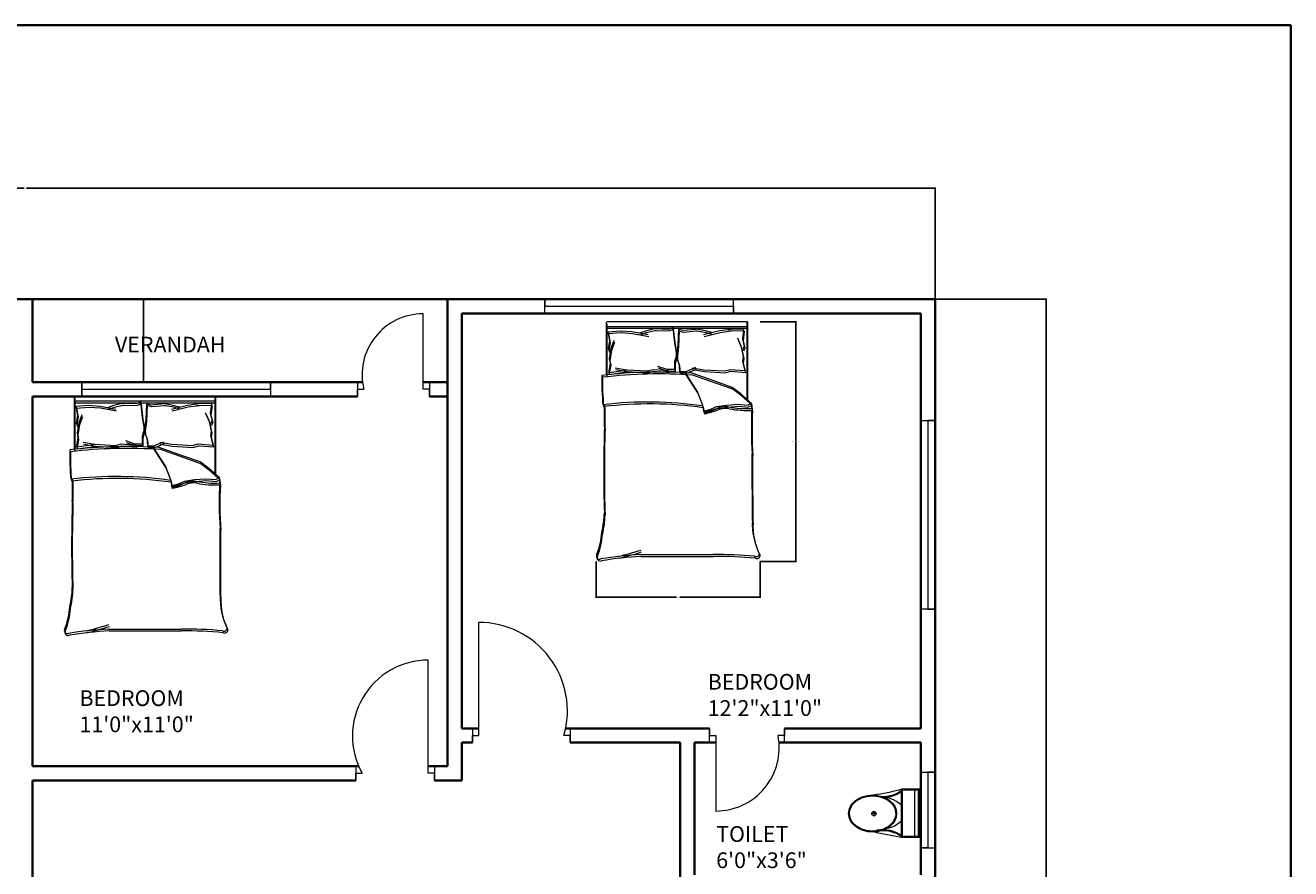
# Model space of a CAD drawing. Units: inches. Extents: x 2234 to 3001, y 1541 to 2386.
# Tile 12 of 12: x 2599 to 3001, y 2118 to 2386. Entities that reach past the tile are written whole.
import ezdxf

# ---------------------------------------------------------------- set-up
doc = ezdxf.new("R2010")
doc.units = ezdxf.units.IN
for name, color, linetype, lineweight in [('A-ANNO-DIMS', 2, 'Continuous', 18), ('A-ANNO-TTLB', 7, 'Continuous', 35), ('A-AREA-IDEN', 7, 'Continuous', 18), ('A-DOOR', 3, 'Continuous', 18), ('A-FLOR-FIXT', 9, 'Continuous', 18), ('A-FURN', 9, 'Continuous', 13), ('A-GLAZ', 4, 'Continuous', 18), ('A-WALL', 7, 'Continuous', 35)]:
    doc.layers.add(name, color=color, linetype=linetype, lineweight=lineweight)
doc.styles.get("Standard").update_dxf_attribs({"font": 'arial.ttf'})
doc.dimstyles.get("Standard").update_dxf_attribs({"dimtxt": 0.18, "dimasz": 0.18, "dimexe": 0.18, "dimexo": 0.0625, "dimgap": 0.09, "dimtad": 0, "dimtih": 1, "dimtoh": 1, "dimdec": 4, "dimzin": 0, "dimdsep": 46, "dimtxsty": 'Standard', "dimcen": 0.09, "dimadec": 0, "dimazin": 0, "dimtfac": 1, "dimtdec": 4, "dimtofl": 0, "dimtmove": 0, "dimatfit": 3, "dimfxl": 1, "dimtolj": 1, "dimtzin": 0, "dimarcsym": 0})

# ---------------------------------------------------------------- blocks, each defined once
blk = doc.blocks.new('A$C31115884')
for p, q in [((283, 498), (223, 498)), ((258, 466), (258, 523)), ((0, 200), (0, 0)), ((520, 200), (0, 200)), ((10, 190), (10, 10)), ((510, 190), (10, 190)), ((510, 10), (510, 190)), ((520, 0), (520, 200)), ((510, 54), (0, 54)), ((10, 10), (510, 10)), ((0, 0), (520, 0))]:
    blk.add_line(p, q)
blk.add_circle((256, 496), 23.6)
for centre, radius, start, end in [((2778, -205), 2807, 165.4549, 171.7133), ((-295, 403), 365, 324.2091, 9.3499), ((-295, 403), 375, 324.2091, 9.3499), ((139, 406), 293, 315.8436, 2.6563), ((806, 403), 365, 170.6501, 215.7909), ((3237, 905), 2807, 188.2867, 194.5451), ((384, 406), 293, 190.2774, 224.1564), ((806, 403), 375, 179.2036, 215.7909)]:
    blk.add_arc(centre, radius, start, end)
blk.add_ellipse((256, 510), major_axis=(0, -261), ratio=0.772727)
blk.add_open_spline([(256, 259), (263, 259), (270, 260), (288, 262), (299, 265), (320, 273), (330, 278), (350, 291), (360, 299), (378, 316), (386, 326), (402, 347), (409, 358), (421, 383), (427, 395), (436, 422), (440, 436), (445, 465), (447, 480), (448, 509), (448, 524), (445, 553), (443, 568), (436, 596), (432, 610), (422, 636), (416, 649), (402, 672), (395, 683), (379, 703), (370, 712), (351, 728), (341, 735), (321, 746), (310, 751), (289, 757), (278, 759), (256, 761), (245, 761), (223, 757), (212, 754), (191, 746), (181, 741), (161, 728), (151, 720), (133, 703), (125, 693), (110, 672), (103, 660), (90, 636), (85, 623), (76, 596), (72, 582), (67, 553), (66, 538), (64, 509), (65, 494), (68, 465), (70, 450), (77, 422), (81, 408), (91, 382), (97, 370), (111, 346), (118, 335), (135, 316), (144, 307), (162, 291), (172, 284), (193, 273), (203, 269), (225, 262), (236, 260), (250, 259), (253, 259), (256, 259)], degree=3, knots=[0, 0, 0, 0, 0.110105, 0.110105, 0.285049, 0.285049, 0.459994, 0.459994, 0.634938, 0.634938, 0.809882, 0.809882, 0.984827, 0.984827, 1.159771, 1.159771, 1.334715, 1.334715, 1.50966, 1.50966, 1.684604, 1.684604, 1.859549, 1.859549, 2.034493, 2.034493, 2.209437, 2.209437, 2.384382, 2.384382, 2.559326, 2.559326, 2.73427, 2.73427, 2.909215, 2.909215, 3.084159, 3.084159, 3.259103, 3.259103, 3.434048, 3.434048, 3.608992, 3.608992, 3.783936, 3.783936, 3.958881, 3.958881, 4.133825, 4.133825, 4.30877, 4.30877, 4.483714, 4.483714, 4.658658, 4.658658, 4.833603, 4.833603, 5.008547, 5.008547, 5.183491, 5.183491, 5.358436, 5.358436, 5.53338, 5.53338, 5.708324, 5.708324, 5.883269, 5.883269, 6.058213, 6.058213, 6.233158, 6.233158, 6.283185, 6.283185, 6.283185, 6.283185])
blk = doc.blocks.new('WIN-60-A')
for p, q in [((0, 60), (4.5, 60)), ((4.5, 60), (2.25, 60)), ((2.25, 60), (2.25, 0)), ((2.25, 0), (0, 0)), ((0, 0), (4.5, 0))]:
    blk.add_line(p, q)
blk = doc.blocks.new('WIN-24-A')
for p, q in [((0, 24), (4.5, 24)), ((4.5, 24), (2.25, 24)), ((2.25, 24), (2.25, 0)), ((2.25, 0), (0, 0)), ((0, 0), (4.5, 0))]:
    blk.add_line(p, q)
blk = doc.blocks.new('WIN-60-B')
for p, q in [((0, 60), (4.5, 60)), ((4.5, 60), (2.25, 60)), ((2.25, 60), (2.25, 0)), ((4.5, 0), (0, 0)), ((2.25, 0), (4.5, 0))]:
    blk.add_line(p, q)
blk = doc.blocks.new('BED-DOUBLE-A')
for p, q in [((3.24, 59.14), (3.24, 76.05)), ((3.24, 59.14), (3.24, 76.05)), ((3.24, 74.62), (47.87, 74.62)), ((3.24, 74.62), (47.87, 74.62)), ((48.08, 76.05), (3.46, 76.05)), ((3.46, 58.54), (3.46, 75.45)), ((3.46, 58.54), (3.46, 75.45)), ((3.46, 74.02), (48.08, 74.02)), ((3.46, 74.02), (48.08, 74.02)), ((3.64, 72.93), (7.64, 73.24)), ((3.64, 72.93), (7.64, 73.24)), ((3.64, 72.95), (4.18, 69.98)), ((3.64, 72.95), (4.18, 69.98)), ((3.85, 72.33), (7.85, 72.64)), ((3.85, 72.33), (7.85, 72.64)), ((7.64, 73.24), (7.74, 73.22)), ((7.64, 73.24), (7.74, 73.22)), ((7.74, 73.22), (11.31, 72.95)), ((7.74, 73.22), (11.31, 72.95)), ((7.85, 72.64), (7.95, 72.62)), ((7.85, 72.64), (7.95, 72.62)), ((7.95, 72.62), (11.52, 72.35)), ((7.95, 72.62), (11.52, 72.35)), ((11.31, 72.95), (16.44, 72.01)), ((11.31, 72.95), (16.44, 72.01)), ((13.87, 72.55), (15.76, 73.22)), ((13.87, 72.55), (15.76, 73.22)), ((14.08, 71.95), (15.97, 72.62)), ((14.08, 71.95), (15.97, 72.62)), ((15.76, 73.22), (18.46, 73.9)), ((15.76, 73.22), (18.46, 73.9)), ((15.97, 72.62), (18.67, 73.3)), ((15.97, 72.62), (18.67, 73.3)), ((18.46, 73.9), (18.76, 73.9)), ((18.46, 73.9), (18.76, 73.9)), ((18.67, 73.3), (18.97, 73.3)), ((18.67, 73.3), (18.97, 73.3)), ((18.76, 73.9), (22.91, 73.76)), ((18.76, 73.9), (22.91, 73.76)), ((18.97, 73.3), (23.12, 73.16)), ((18.97, 73.3), (23.12, 73.16)), ((22.91, 73.76), (24.26, 74.3)), ((22.91, 73.76), (24.26, 74.3)), ((23.12, 73.16), (24.47, 73.7)), ((23.12, 73.16), (24.47, 73.7)), ((24.26, 74.3), (24.8, 69.31)), ((24.26, 74.3), (24.8, 69.31)), ((24.47, 73.7), (25.01, 68.71)), ((24.47, 73.7), (25.01, 68.71)), ((26.12, 73.72), (25.9, 68.7)), ((26.12, 73.72), (25.9, 68.7)), ((26.34, 73.12), (26.11, 68.1)), ((26.34, 73.12), (26.11, 68.1)), ((27.5, 73.27), (26.12, 73.72)), ((27.5, 73.27), (26.12, 73.72)), ((27.72, 72.67), (26.34, 73.12)), ((27.72, 72.67), (26.34, 73.12)), ((31.64, 73.66), (27.5, 73.27)), ((31.64, 73.66), (27.5, 73.27)), ((31.85, 73.06), (27.72, 72.67)), ((31.85, 73.06), (27.72, 72.67)), ((31.94, 73.68), (31.64, 73.66)), ((31.94, 73.68), (31.64, 73.66)), ((32.15, 73.08), (31.85, 73.06)), ((32.15, 73.08), (31.85, 73.06)), ((34.67, 73.17), (31.94, 73.68)), ((34.67, 73.17), (31.94, 73.68)), ((34.89, 72.58), (32.15, 73.08)), ((34.89, 72.58), (32.15, 73.08)), ((39.14, 73.18), (34.08, 71.92)), ((39.14, 73.18), (34.08, 71.92)), ((39.35, 72.58), (34.29, 71.32)), ((39.35, 72.58), (34.29, 71.32)), ((36.6, 72.62), (34.67, 73.17)), ((36.6, 72.62), (34.67, 73.17)), ((36.82, 72.02), (34.89, 72.58)), ((36.82, 72.02), (34.89, 72.58)), ((42.68, 73.67), (39.14, 73.18)), ((42.68, 73.67), (39.14, 73.18)), ((42.9, 73.08), (39.35, 72.58)), ((42.9, 73.08), (39.35, 72.58)), ((46.79, 73.66), (41.75, 73.75)), ((41.75, 73.75), (42.68, 73.67)), ((46.79, 73.66), (41.75, 73.75)), ((41.75, 73.75), (42.68, 73.67)), ((47.01, 73.06), (41.96, 73.15)), ((41.96, 73.15), (42.9, 73.08)), ((47, 73.06), (41.96, 73.15)), ((41.96, 73.15), (42.9, 73.08)), ((46.79, 73.66), (46.44, 70.66)), ((46.79, 73.66), (46.44, 70.66)), ((47.01, 73.06), (46.65, 70.07)), ((47, 73.06), (46.65, 70.07)), ((47.87, 76.05), (47.87, 51.2)), ((47.87, 76.05), (47.87, 51.2)), ((48.08, 76.05), (48.08, 75.45)), ((48.08, 75.45), (48.08, 50.6)), ((48.08, 75.45), (48.08, 50.6)), ((4.18, 69.98), (3.77, 67.55)), ((4.18, 69.98), (3.77, 67.55)), ((3.85, 72.35), (4.39, 69.38)), ((3.85, 72.35), (4.39, 69.38)), ((4.39, 69.38), (3.98, 66.95)), ((4.39, 69.38), (3.98, 66.95)), ((4.72, 67.69), (5.66, 70.25)), ((4.72, 67.69), (5.66, 70.25)), ((4.93, 67.09), (5.87, 69.65)), ((4.93, 67.09), (5.87, 69.65)), ((11.52, 72.35), (16.65, 71.41)), ((11.52, 72.35), (16.65, 71.41)), ((24.8, 69.31), (25.34, 66.34)), ((24.8, 69.31), (25.34, 66.34)), ((25.01, 68.71), (25.55, 65.74)), ((25.01, 68.71), (25.55, 65.74)), ((25.9, 68.7), (25.54, 65.7)), ((25.9, 68.7), (25.54, 65.7)), ((46.04, 68.34), (44.94, 70.84)), ((46.04, 68.34), (44.94, 70.84)), ((46.26, 67.74), (45.15, 70.24)), ((46.26, 67.74), (45.15, 70.24)), ((46.44, 70.66), (46.99, 68.26)), ((46.44, 70.66), (46.99, 68.26)), ((46.65, 70.07), (47.21, 67.66)), ((46.65, 70.07), (47.21, 67.66)), ((3.77, 67.55), (4.31, 66.61)), ((3.77, 67.55), (4.31, 66.61)), ((3.98, 66.95), (4.52, 66.01)), ((3.98, 66.95), (4.52, 66.01)), ((4.18, 64.31), (4.72, 67.69)), ((4.18, 64.31), (4.72, 67.69)), ((4.39, 63.71), (4.93, 67.09)), ((4.39, 63.71), (4.93, 67.09)), ((25.34, 65.12), (24.8, 63.37)), ((25.34, 65.12), (24.8, 63.37)), ((25.55, 64.52), (25.01, 62.77)), ((25.55, 64.52), (25.01, 62.77)), ((25.34, 66.34), (25.34, 65.12)), ((25.34, 66.34), (25.34, 65.12)), ((25.54, 65.7), (25.62, 64.49)), ((25.54, 65.7), (25.62, 64.49)), ((25.55, 65.74), (25.55, 64.52)), ((25.55, 65.74), (25.55, 64.52)), ((25.62, 64.49), (26.27, 62.77)), ((25.62, 64.49), (26.27, 62.77)), ((26.11, 68.1), (25.76, 65.11)), ((26.11, 68.1), (25.76, 65.11)), ((25.76, 65.11), (25.83, 63.89)), ((25.76, 65.11), (25.83, 63.89)), ((46.79, 65), (46.04, 68.34)), ((46.79, 65), (46.04, 68.34)), ((47.01, 64.41), (46.26, 67.74)), ((47, 64.41), (46.26, 67.74)), ((46.99, 68.26), (46.51, 67.28)), ((46.99, 68.26), (46.51, 67.28)), ((46.61, 63.5), (46.79, 65)), ((46.62, 63.5), (46.79, 65)), ((47.21, 67.66), (46.73, 66.69)), ((47.21, 67.66), (46.73, 66.69)), ((46.83, 62.91), (47.01, 64.41)), ((46.83, 62.91), (47, 64.41)), ((3.91, 59.86), (4.45, 62.83)), ((3.91, 59.86), (4.45, 62.83)), ((8.67, 60.53), (3.91, 59.86)), ((8.67, 60.53), (3.91, 59.86)), ((4.12, 59.26), (4.66, 62.23)), ((4.12, 59.26), (4.66, 62.23)), ((4.45, 62.83), (4.18, 64.31)), ((4.45, 62.83), (4.18, 64.31)), ((4.66, 62.23), (4.39, 63.71)), ((4.66, 62.23), (4.39, 63.71)), ((5.96, 61.45), (9.72, 60.83)), ((5.96, 61.45), (9.72, 60.83)), ((6.17, 60.86), (9.94, 60.24)), ((6.17, 60.86), (9.94, 60.24)), ((9.72, 60.83), (8.67, 60.53)), ((9.72, 60.83), (8.67, 60.53)), ((9.72, 60.83), (16.27, 60.43)), ((9.72, 60.83), (16.27, 60.43)), ((16.27, 60.43), (18.1, 60.95)), ((16.27, 60.43), (18.1, 60.95)), ((16.48, 59.83), (18.31, 60.35)), ((16.48, 59.83), (18.31, 60.35)), ((18.1, 60.95), (22.89, 60.57)), ((18.1, 60.95), (22.89, 60.57)), ((18.31, 60.35), (23.1, 59.98)), ((18.31, 60.35), (23.1, 59.98)), ((22.51, 60.86), (19.57, 61.88)), ((22.51, 60.86), (19.57, 61.88)), ((22.72, 60.27), (19.78, 61.28)), ((22.72, 60.27), (19.78, 61.28)), ((24.8, 60.86), (22.51, 60.86)), ((24.8, 60.86), (22.51, 60.86)), ((24.8, 63.37), (24.8, 60.86)), ((24.8, 63.37), (24.8, 60.86)), ((25.01, 62.77), (25.01, 60.27)), ((25.01, 62.77), (25.01, 60.27)), ((25.83, 63.89), (26.48, 62.18)), ((25.83, 63.89), (26.48, 62.18)), ((26.27, 62.77), (26.42, 60.27)), ((26.27, 62.77), (26.42, 60.27)), ((26.42, 60.27), (28.71, 60.42)), ((26.42, 60.27), (28.71, 60.42)), ((26.48, 62.18), (26.64, 59.68)), ((26.48, 62.18), (26.64, 59.68)), ((28.71, 60.42), (31.58, 61.62)), ((28.71, 60.42), (31.58, 61.62)), ((28.93, 59.82), (31.79, 61.02)), ((28.93, 59.82), (31.79, 61.02)), ((30.41, 61.45), (34.17, 60.83)), ((30.41, 61.45), (34.17, 60.83)), ((30.62, 60.86), (34.38, 60.24)), ((30.62, 60.86), (34.38, 60.24)), ((34.17, 60.83), (40.72, 60.43)), ((34.17, 60.83), (40.72, 60.43)), ((40.72, 60.43), (42.55, 60.95)), ((40.72, 60.43), (42.55, 60.95)), ((40.93, 59.83), (42.76, 60.35)), ((40.93, 59.83), (42.76, 60.35)), ((42.55, 60.95), (47.34, 60.57)), ((42.55, 60.95), (47.34, 60.57)), ((42.76, 60.35), (47.55, 59.98)), ((42.76, 60.35), (47.55, 59.98)), ((47.34, 60.57), (46.61, 63.5)), ((47.34, 60.57), (46.62, 63.5)), ((47.55, 59.98), (46.83, 62.91)), ((47.55, 59.98), (46.83, 62.91)), ((8.88, 59.93), (4.12, 59.26)), ((8.88, 59.93), (4.12, 59.26)), ((9.94, 60.24), (8.88, 59.93)), ((9.94, 60.24), (8.88, 59.93)), ((9.94, 60.24), (16.48, 59.83)), ((9.94, 60.24), (16.48, 59.83)), ((25.01, 60.27), (22.72, 60.27)), ((25.01, 60.27), (22.72, 60.27)), ((26.64, 59.68), (28.93, 59.82)), ((26.64, 59.68), (28.93, 59.82)), ((28.25, 59.82), (32.17, 53.75)), ((28.25, 59.82), (32.17, 53.75)), ((28.47, 59.22), (32.38, 53.16)), ((28.47, 59.22), (32.38, 53.16)), ((37.95, 57.08), (30.17, 59.82)), ((37.95, 57.08), (30.17, 59.82)), ((38.16, 56.48), (30.38, 59.22)), ((38.16, 56.48), (30.38, 59.22)), ((34.38, 60.24), (40.93, 59.83)), ((34.38, 60.24), (40.93, 59.83)), ((43.16, 55.2), (37.95, 57.08)), ((43.16, 55.2), (37.95, 57.08)), ((43.37, 54.6), (38.16, 56.48)), ((43.37, 54.6), (38.16, 56.48)), ((32.17, 53.75), (33.76, 49.56)), ((32.17, 53.75), (33.76, 49.56)), ((32.38, 53.16), (33.97, 48.97)), ((32.38, 53.16), (33.97, 48.97)), ((45.91, 53.18), (43.16, 55.2)), ((45.9, 53.18), (43.16, 55.2)), ((46.12, 52.58), (43.37, 54.6)), ((46.12, 52.58), (43.37, 54.6)), ((49.36, 50.14), (45.9, 53.18)), ((49.37, 50.14), (45.91, 53.18)), ((49.58, 49.54), (46.12, 52.58)), ((49.58, 49.54), (46.12, 52.58)), ((33.76, 49.56), (34.05, 47.68)), ((33.76, 49.56), (34.05, 47.68)), ((33.97, 48.97), (34.26, 47.09)), ((33.97, 48.97), (34.26, 47.09)), ((36.36, 48.26), (38.24, 49.13)), ((36.36, 48.26), (38.24, 49.13)), ((36.57, 47.66), (38.45, 48.53)), ((36.57, 47.66), (38.45, 48.53)), ((38.24, 49.13), (41.42, 49.56)), ((38.24, 49.13), (41.42, 49.56)), ((38.45, 48.53), (41.64, 48.97)), ((38.45, 48.53), (41.64, 48.97)), ((41.42, 49.56), (45.04, 49.85)), ((41.42, 49.56), (45.04, 49.85)), ((41.64, 48.97), (45.25, 49.25)), ((41.64, 48.97), (45.25, 49.25)), ((45.04, 49.85), (47.93, 49.56)), ((45.04, 49.85), (47.93, 49.56)), ((45.25, 49.25), (48.14, 48.97)), ((45.25, 49.25), (48.14, 48.97)), ((47.93, 49.56), (49.37, 50.14)), ((47.93, 49.56), (49.36, 50.14)), ((48.14, 48.97), (49.58, 49.54)), ((48.14, 48.97), (49.58, 49.54)), ((49.44, 48.51), (49.36, 50.14, 3.61)), ((49.44, 48.51), (49.37, 50.14, 3.61)), ((49.65, 47.91), (49.58, 49.54, 3.61)), ((49.65, 47.91), (49.58, 49.54, 3.61)), ((34.05, 47.68), (36.36, 48.26)), ((34.05, 47.68), (36.36, 48.26)), ((34.26, 47.09), (36.57, 47.66)), ((34.26, 47.09), (36.57, 47.66)), ((14.07, 2.05), (37.05, 2.05)), ((14.07, 2.05), (37.05, 2.05)), ((14.28, 1.46), (37.26, 1.46)), ((14.28, 1.46), (37.26, 1.46))]:
    blk.add_line(p, q)
for centre, radius, start, end in [((79.52, 57.28), 77.79, 178.7218, 185.604), ((79.52, 57.28), 77.79, 178.7218, 185.604), ((19.94, -93.94), 154.04, 86.0865, 96.7821), ((19.94, -93.94), 154.04, 86.0865, 96.7821), ((79.73, 56.69), 77.79, 178.7218, 185.604), ((79.73, 56.69), 77.79, 178.7218, 185.604), ((20.16, -94.54), 154.04, 86.0865, 96.7821), ((20.16, -94.54), 154.04, 86.0865, 96.7821), ((16.58, -69.91), 120.47, 81.7845, 96.9006), ((16.58, -69.91), 120.47, 81.7845, 96.9006), ((16.79, -70.51), 120.47, 81.7845, 96.9006), ((16.79, -70.51), 120.47, 81.7845, 96.9006), ((-156.22, 46.94), 158.84, 358.4762, 1.0082), ((-156.22, 46.94), 158.84, 358.4762, 1.0082), ((-156.01, 46.34), 158.84, 358.4762, 1.0082), ((-156.01, 46.34), 158.84, 358.4762, 1.0082), ((29.09, 74.66), 27.69, 280.6617, 289.8806), ((29.09, 74.66), 27.69, 280.6617, 289.8806), ((40.85, 43.3), 5.81, 78.6608, 113.7384), ((40.85, 43.3), 5.81, 78.6608, 113.7384), ((41.06, 42.71), 5.81, 78.6608, 113.7384), ((41.06, 42.71), 5.81, 78.6608, 113.7384), ((47.93, 82.26), 33.79, 259.8763, 272.5657), ((47.93, 82.26), 33.79, 259.8763, 272.5657), ((48.14, 81.67), 33.79, 259.8763, 272.5657), ((48.14, 81.67), 33.79, 259.8763, 272.5657), ((170.19, 42.14), 120.92, 176.9791, 183.8365), ((170.19, 42.14), 120.92, 176.9791, 183.8365), ((34.21, 47.63), 0.172, 160.2464, 271.1377), ((34.21, 47.63), 0.172, 160.2464, 271.1377), ((34.42, 47.03), 0.172, 160.2464, 271.1377), ((34.42, 47.03), 0.172, 160.2464, 271.1377), ((29.3, 74.07), 27.69, 280.6617, 289.8806), ((29.3, 74.07), 27.69, 280.6617, 289.8806), ((170.4, 41.54), 120.92, 176.9791, 183.8365), ((170.4, 41.54), 120.92, 176.9791, 183.8365), ((452.7, 28.79), 450.36, 178.2277, 181.7185), ((452.7, 28.79), 450.36, 178.2277, 181.7185), ((452.91, 28.19), 450.36, 178.2277, 181.7185), ((452.91, 28.19), 450.36, 178.2277, 181.7185), ((-4210.02, 12.72), 4259.62, 0.00217, 0.28689), ((-4210.02, 12.72), 4259.62, 0.00217, 0.28689), ((-4209.81, 12.12), 4259.62, 0.00217, 0.28689), ((-4209.81, 12.12), 4259.62, 0.00217, 0.28689), ((-25.12, 15.81), 27.67, 346.0648, 358.9113), ((-25.12, 15.81), 27.67, 346.0648, 358.9113), ((-24.9, 15.21), 27.67, 346.0648, 358.9113), ((-24.9, 15.21), 27.67, 346.0648, 358.9113), ((71.11, 11.93), 21.54, 177.4714, 206.4681), ((71.11, 11.93), 21.54, 177.4714, 206.4681), ((71.32, 11.33), 21.54, 177.4714, 206.4681), ((71.32, 11.33), 21.54, 177.4714, 206.4681), ((-20.22, 10.43), 22, 337.9751, 356.652), ((-20.22, 10.43), 22, 337.9751, 356.652), ((-20.01, 9.83), 22, 337.9751, 356.652), ((-20.01, 9.83), 22, 337.9751, 356.652), ((1.02, 1.61), 1.02, 146.1736, 293.4781), ((1.02, 1.61), 1.02, 146.1736, 293.4781), ((1.23, 1.01), 1.02, 146.1736, 293.4781), ((1.23, 1.01), 1.02, 146.1736, 293.4781), ((20.01, -111.48), 113.69, 92.9958, 99.4091), ((20.01, -111.48), 113.69, 92.9958, 99.4091), ((20.22, -112.08), 113.69, 92.9958, 99.4091), ((20.22, -112.08), 113.69, 92.9958, 99.4091), ((-16.08, 98.19), 99.41, 283.3832, 287.7053), ((-16.08, 98.19), 99.41, 283.3832, 287.7053), ((-15.87, 97.59), 99.41, 283.3832, 287.7053), ((-15.87, 97.59), 99.41, 283.3832, 287.7053), ((38.43, -122.16), 124.23, 84.4998, 90.6351), ((38.43, -122.16), 124.23, 84.4998, 90.6351), ((38.64, -122.76), 124.23, 84.4998, 90.6351), ((38.64, -122.76), 124.23, 84.4998, 90.6351), ((50.81, 2.4), 1.03, 242.6588, 356.02), ((50.8, 2.4), 1.03, 242.6588, 356.02), ((51.02, 1.81), 1.03, 242.6588, 356.02), ((51.02, 1.81), 1.03, 242.6588, 356.02)]:
    blk.add_arc(centre, radius, start, end)
blk = doc.blocks.new('*D35')
at = {"layer": 'A-ANNO-DIMS', "color": 0, "lineweight": -2, "transparency": 16777216}
for p, q in [((2832.68, 2291.4), (2844.22, 2291.4)), ((2844.04, 2291.22), (2844.04, 2253.51)), ((2844.04, 2215.44), (2844.04, 2253.15)), ((2832.68, 2215.26), (2844.22, 2215.26))]:
    blk.add_line(p, q, dxfattribs=at)
at = {"layer": 'A-ANNO-DIMS', "color": 0, "transparency": 16777216}
for points in [[(2844.01, 2291.22), (2844.07, 2291.22), (2844.04, 2291.4)], [(2844.01, 2215.44), (2844.07, 2215.44), (2844.04, 2215.26)]]:
    blk.add_solid(points, dxfattribs=at)
at = {"layer": 'Defpoints', "color": 0, "transparency": 16777216}
for p in [(2832.62, 2291.4), (2844.04, 2291.4), (2832.62, 2215.26)]:
    blk.add_point(p, dxfattribs=at)
at = {"layer": 'A-ANNO-DIMS', "color": 0, "transparency": 16777216, "insert": (2844.04, 2253.33), "char_height": 0.18, "attachment_point": 5}
blk.add_mtext('\\A1;DOUBLE BED A 76 TYP.', dxfattribs=at)
blk = doc.blocks.new('*D36')
at = {"layer": 'A-ANNO-DIMS', "color": 0, "lineweight": -2, "transparency": 16777216}
for p, q in [((2780.49, 2215.19), (2780.49, 2203.66)), ((2832.62, 2215.19), (2832.62, 2203.66)), ((2780.67, 2203.84), (2806.03, 2203.84)), ((2832.44, 2203.84), (2807.09, 2203.84))]:
    blk.add_line(p, q, dxfattribs=at)
at = {"layer": 'A-ANNO-DIMS', "color": 0, "transparency": 16777216}
for points in [[(2780.67, 2203.87), (2780.67, 2203.81), (2780.49, 2203.84)], [(2832.44, 2203.87), (2832.44, 2203.81), (2832.62, 2203.84)]]:
    blk.add_solid(points, dxfattribs=at)
at = {"layer": 'Defpoints', "color": 0, "transparency": 16777216}
for p in [(2780.49, 2215.26), (2832.62, 2215.26), (2832.62, 2203.84)]:
    blk.add_point(p, dxfattribs=at)
at = {"layer": 'A-ANNO-DIMS', "color": 0, "transparency": 16777216, "insert": (2806.56, 2203.84), "char_height": 0.18, "attachment_point": 5}
blk.add_mtext('\\A1;52 TYP.', dxfattribs=at)
blk = doc.blocks.new('*D61')
at = {"layer": 'A-ANNO-DIMS', "color": 0, "lineweight": -2, "transparency": 16777216}
for p, q in [((2309.75, 2298.67), (2309.75, 2334.14)), ((2309.93, 2333.96), (2598.61, 2333.96)), ((2888.07, 2333.96), (2599.4, 2333.96)), ((2888.25, 2298.67), (2888.25, 2334.14))]:
    blk.add_line(p, q, dxfattribs=at)
at = {"layer": 'A-ANNO-DIMS', "color": 0, "transparency": 16777216}
for points in [[(2309.93, 2333.99), (2309.93, 2333.93), (2309.75, 2333.96)], [(2888.07, 2333.99), (2888.07, 2333.93), (2888.25, 2333.96)]]:
    blk.add_solid(points, dxfattribs=at)
at = {"layer": 'Defpoints', "color": 0, "transparency": 16777216}
for p in [(2888.25, 2333.96), (2309.75, 2298.61), (2888.25, 2298.61)]:
    blk.add_point(p, dxfattribs=at)
at = {"layer": 'A-ANNO-DIMS', "color": 0, "transparency": 16777216, "insert": (2599, 2333.96), "char_height": 0.18, "attachment_point": 5}
blk.add_mtext('\\A1;578.5', dxfattribs=at)
blk = doc.blocks.new('*D62')
at = {"layer": 'A-ANNO-DIMS', "color": 0, "lineweight": -2, "transparency": 16777216}
for p, q in [((2888.32, 2298.61), (2923.78, 2298.61)), ((2923.6, 2298.43), (2923.6, 2000.54)), ((2923.6, 1702.29), (2923.6, 2000.18)), ((2888.32, 1702.11), (2923.78, 1702.11))]:
    blk.add_line(p, q, dxfattribs=at)
at = {"layer": 'A-ANNO-DIMS', "color": 0, "transparency": 16777216}
for points in [[(2923.57, 2298.43), (2923.63, 2298.43), (2923.6, 2298.61)], [(2923.57, 1702.29), (2923.63, 1702.29), (2923.6, 1702.11)]]:
    blk.add_solid(points, dxfattribs=at)
at = {"layer": 'Defpoints', "color": 0, "transparency": 16777216}
for p in [(2888.25, 2298.61), (2923.6, 2298.61), (2888.25, 1702.11)]:
    blk.add_point(p, dxfattribs=at)
at = {"layer": 'A-ANNO-DIMS', "color": 0, "transparency": 16777216, "insert": (2923.6, 2000.36), "char_height": 0.18, "attachment_point": 5}
blk.add_mtext('\\A1;596.5', dxfattribs=at)
blk = doc.blocks.new('*D67')
at = {"layer": 'A-ANNO-DIMS', "color": 0, "lineweight": -2, "transparency": 16777216}
for p, q in [((2601.32, 2298.61), (2636.78, 2298.61)), ((2636.6, 2298.43), (2636.6, 2285.6)), ((2636.6, 2272.4), (2636.6, 2285.23)), ((2601.32, 2272.22), (2636.78, 2272.22))]:
    blk.add_line(p, q, dxfattribs=at)
at = {"layer": 'A-ANNO-DIMS', "color": 0, "transparency": 16777216}
for points in [[(2636.57, 2298.43), (2636.63, 2298.43), (2636.6, 2298.61)], [(2636.57, 2272.4), (2636.63, 2272.4), (2636.6, 2272.22)]]:
    blk.add_solid(points, dxfattribs=at)
at = {"layer": 'Defpoints', "color": 0, "transparency": 16777216}
for p in [(2601.25, 2298.61), (2601.25, 2272.22), (2636.6, 2272.22)]:
    blk.add_point(p, dxfattribs=at)
at = {"layer": 'A-ANNO-DIMS', "color": 0, "transparency": 16777216, "insert": (2636.6, 2285.41), "char_height": 0.18, "attachment_point": 5}
blk.add_mtext('\\A1;26.39', dxfattribs=at)

msp = doc.modelspace()

# ---------------------------------------------------------------- linework, layer by layer
at = {"layer": 'A-ANNO-TTLB'}
msp.add_lwpolyline([(2233.5367, 2385.7012), (3001.3383, 2385.7012), (3001.3383, 1541.435), (2233.5367, 1541.435)], close=True, dxfattribs=at)
at = {"layer": 'A-DOOR'}
for p, q in [((2725.479, 2269.9685), (2725.479, 2293.9685)), ((2704.6613, 2272.2185), (2704.6613, 2267.7185)), ((2704.6613, 2267.7185), (2704.6613, 2269.9685)), ((2704.6613, 2269.9685), (2706.6613, 2269.9685)), ((2727.479, 2269.9685), (2725.479, 2269.9685)), ((2727.479, 2272.2185), (2727.479, 2267.7185)), ((2727.479, 2267.7185), (2727.479, 2269.9685)), ((2743.1877, 2159.861), (2743.1877, 2195.861)), ((2727.1204, 2147.861), (2727.1204, 2183.861)), ((2741.1877, 2162.111), (2741.1877, 2157.611)), ((2772.2799, 2162.111), (2772.2799, 2157.611)), ((2816.5683, 2157.611), (2816.5683, 2162.111)), ((2816.5683, 2162.111), (2816.5683, 2159.861)), ((2840.3413, 2157.611), (2840.3413, 2162.111)), ((2840.3413, 2162.111), (2840.3413, 2159.861)), ((2741.1877, 2157.611), (2741.1877, 2159.861)), ((2741.1877, 2159.861), (2743.1877, 2159.861)), ((2741.1877, 2157.611), (2741.1877, 2157.611)), ((2772.2799, 2159.861), (2770.2799, 2159.861)), ((2772.2799, 2157.611), (2772.2799, 2159.861)), ((2816.5683, 2159.861), (2818.5683, 2159.861)), ((2818.5683, 2159.861), (2818.5683, 2135.861)), ((2840.3413, 2159.861), (2838.3413, 2159.861)), ((2704.1426, 2150.111), (2704.1426, 2145.611)), ((2729.1204, 2150.111), (2729.1204, 2145.611)), ((2704.1426, 2145.611), (2704.1426, 2147.861)), ((2704.1426, 2147.861), (2706.1426, 2147.861)), ((2729.1204, 2147.861), (2727.1204, 2147.861)), ((2729.1204, 2145.611), (2729.1204, 2147.861))]:
    msp.add_line(p, q, dxfattribs=at)
for centre, radius, start, end in [((2725.479, 2274.5913), 19.3772, 90, 193.802081), ((2743.1877, 2167.6667), 28.1943, 343.927438, 90), ((2727.1204, 2159.7489), 24.1121, 90, 209.539718), ((2818.5683, 2156.0063), 20.1452, 270, 11.031501)]:
    msp.add_arc(centre, radius, start, end, dxfattribs=at)
at = {"layer": 'A-GLAZ'}
msp.add_line((2616.9992, 2272.2185), (2616.9992, 2267.7185), dxfattribs=at)
at = {"layer": 'A-WALL'}
for p, q in [((2464.7534, 2298.611), (2733.2534, 2298.611)), ((2596.7534, 2298.611), (2601.2534, 2298.611)), ((2601.2534, 2298.611), (2601.2534, 2272.2185)), ((2733.2534, 2298.611), (2733.2534, 2157.611)), ((2733.2534, 2298.611), (2888.2534, 2298.611)), ((2888.2534, 2298.611), (2888.2534, 1702.111)), ((2737.7534, 2294.111), (2737.7534, 2162.111)), ((2737.7534, 2294.111), (2883.7534, 2294.111)), ((2883.7534, 2294.111), (2883.7534, 2162.111)), ((2733.2534, 2282.111), (2733.2534, 2150.111)), ((2601.2534, 2277.611), (2601.2534, 2272.2185)), ((2601.2534, 2272.2185), (2706.2476, 2272.2185)), ((2725.479, 2272.2185), (2733.2534, 2272.2185)), ((2601.2534, 2267.7185), (2704.6613, 2267.7185)), ((2601.2534, 2267.7185), (2601.2534, 2150.111)), ((2727.479, 2267.7185), (2733.2534, 2267.7185)), ((2737.7534, 2162.111), (2743.1877, 2162.111)), ((2770.8292, 2162.111), (2816.5683, 2162.111)), ((2811.7534, 2162.111), (2807.2534, 2162.111)), ((2840.3413, 2162.111), (2883.7534, 2162.111)), ((2737.7534, 2157.611), (2741.1877, 2157.611)), ((2737.7534, 2145.611), (2737.7534, 2157.611)), ((2772.2799, 2157.611), (2807.2534, 2157.611)), ((2807.2534, 2157.611), (2807.2534, 2107.6086)), ((2811.7534, 2157.611), (2818.5683, 2157.611)), ((2811.7534, 2115.611), (2811.7534, 2157.611)), ((2838.6495, 2157.611), (2883.7534, 2157.611)), ((2883.7534, 2157.611), (2883.7534, 2115.611)), ((2705.0183, 2150.111), (2601.2534, 2150.111)), ((2733.2534, 2150.111), (2727.1204, 2150.111)), ((2601.2534, 2145.611), (2704.1426, 2145.611)), ((2601.2534, 2145.611), (2601.2534, 2004.611)), ((2729.1204, 2145.611), (2737.7534, 2145.611))]:
    msp.add_line(p, q, dxfattribs=at)

# ---------------------------------------------------------------- block references
at = {"layer": 'A-FLOR-FIXT', "xscale": 0.0292470664339069, "yscale": 0.0292470664339069, "zscale": 0.0292470664339069, "rotation": 89.99999999999999}
msp.add_blockref('A$C31115884', (2883.3221, 2127.5818), dxfattribs=at)
at = {"layer": 'A-FURN'}
for p in [(2780.5758, 2215.3549), (2611.3897, 2191.6708)]:
    msp.add_blockref('BED-DOUBLE-A', p, dxfattribs=at)
at = {"layer": 'A-GLAZ', "rotation": 90}
for name, p in [('WIN-60-A', (2824.1492, 2294.1106)), ('WIN-60-B', (2676.9995, 2267.7181))]:
    msp.add_blockref(name, p, dxfattribs=at)
at = {"layer": 'A-GLAZ'}
for name, p in [('WIN-60-B', (2883.753, 2200.044)), ('WIN-24-A', (2883.753, 2124.188))]:
    msp.add_blockref(name, p, dxfattribs=at)

# ---------------------------------------------------------------- texts
at = {"layer": 'A-AREA-IDEN', "char_height": 5, "attachment_point": 1}
for s, width, insert in [('VERANDAH', 107.840646, (2627.5021, 2286.6671)), ('BEDROOM\\P12\'2"x11\'0"', 154.732428, (2815.9725, 2179.4572)), ('BEDROOM\\P11\'0"x11\'0"', 143.404712, (2616.2193, 2174.2588)), ('TOILET\\P6\'0"x3\'6"', 87.716683, (2818.6797, 2131.0638))]:
    msp.add_mtext_dynamic_manual_height_columns(s, width=width, gutter_width=12.5, heights=[0], dxfattribs=dict(at, insert=insert))

# ---------------------------------------------------------------- dimensions: what is measured, and where the dimension line sits
at = {"layer": 'A-ANNO-DIMS'}
dim = msp.add_linear_dim(base=(2888.2534, 2333.961), p1=(2309.7534, 2298.611), p2=(2888.2534, 2298.611), dimstyle='Standard', override={"dimdec": 1, "dimlfac": 1, "dimrnd": 0, "dimzin": 0, "dimdsep": 46, "dimlunit": 2}, dxfattribs=at)
dim.commit()
dim.dimension.update_dxf_attribs({"geometry": '*D61', "text_midpoint": (2599.0034, 2333.961)})
for base, p1, p2, angle, override, picture, middle in [((2636.6034, 2272.2185), (2601.2534, 2298.611), (2601.2534, 2272.2185), 270, {"dimdec": 2, "dimlfac": 1, "dimrnd": 0, "dimzin": 0, "dimdsep": 46, "dimlunit": 2}, '*D67', (2636.6034, 2285.4148)), ((2923.6034, 2298.611), (2888.2534, 1702.111), (2888.2534, 2298.611), 90, {"dimdec": 1, "dimlfac": 1, "dimrnd": 0, "dimzin": 0, "dimdsep": 46, "dimlunit": 2}, '*D62', (2923.6034, 2000.361))]:
    dim = msp.add_linear_dim(base=base, p1=p1, p2=p2, angle=angle, dimstyle='Standard', override=override, dxfattribs=at)
    dim.commit()
    dim.dimension.update_dxf_attribs({"geometry": picture, "text_midpoint": middle})
dim = msp.add_linear_dim(base=(2844.0428, 2291.4026), p1=(2832.621, 2215.2569), p2=(2832.621, 2291.4026), angle=90, text='DOUBLE BED A <> TYP.', dimstyle='Standard', override={"dimdec": 0, "dimlfac": 1, "dimrnd": 0, "dimzin": 0, "dimdsep": 46, "dimlunit": 2}, dxfattribs=at)
dim.commit()
dim.dimension.update_dxf_attribs({"geometry": '*D35', "text_midpoint": (2844.0428, 2253.3298)})
dim = msp.add_linear_dim(base=(2832.621, 2203.835), p1=(2780.495, 2215.2569), p2=(2832.621, 2215.2569), text='<> TYP.', dimstyle='Standard', override={"dimdec": 0, "dimlfac": 1, "dimrnd": 0, "dimzin": 0, "dimdsep": 46, "dimlunit": 2}, dxfattribs=at)
dim.commit()
dim.dimension.update_dxf_attribs({"geometry": '*D36', "text_midpoint": (2806.558, 2203.835)})

doc.saveas('drawing.dxf')
